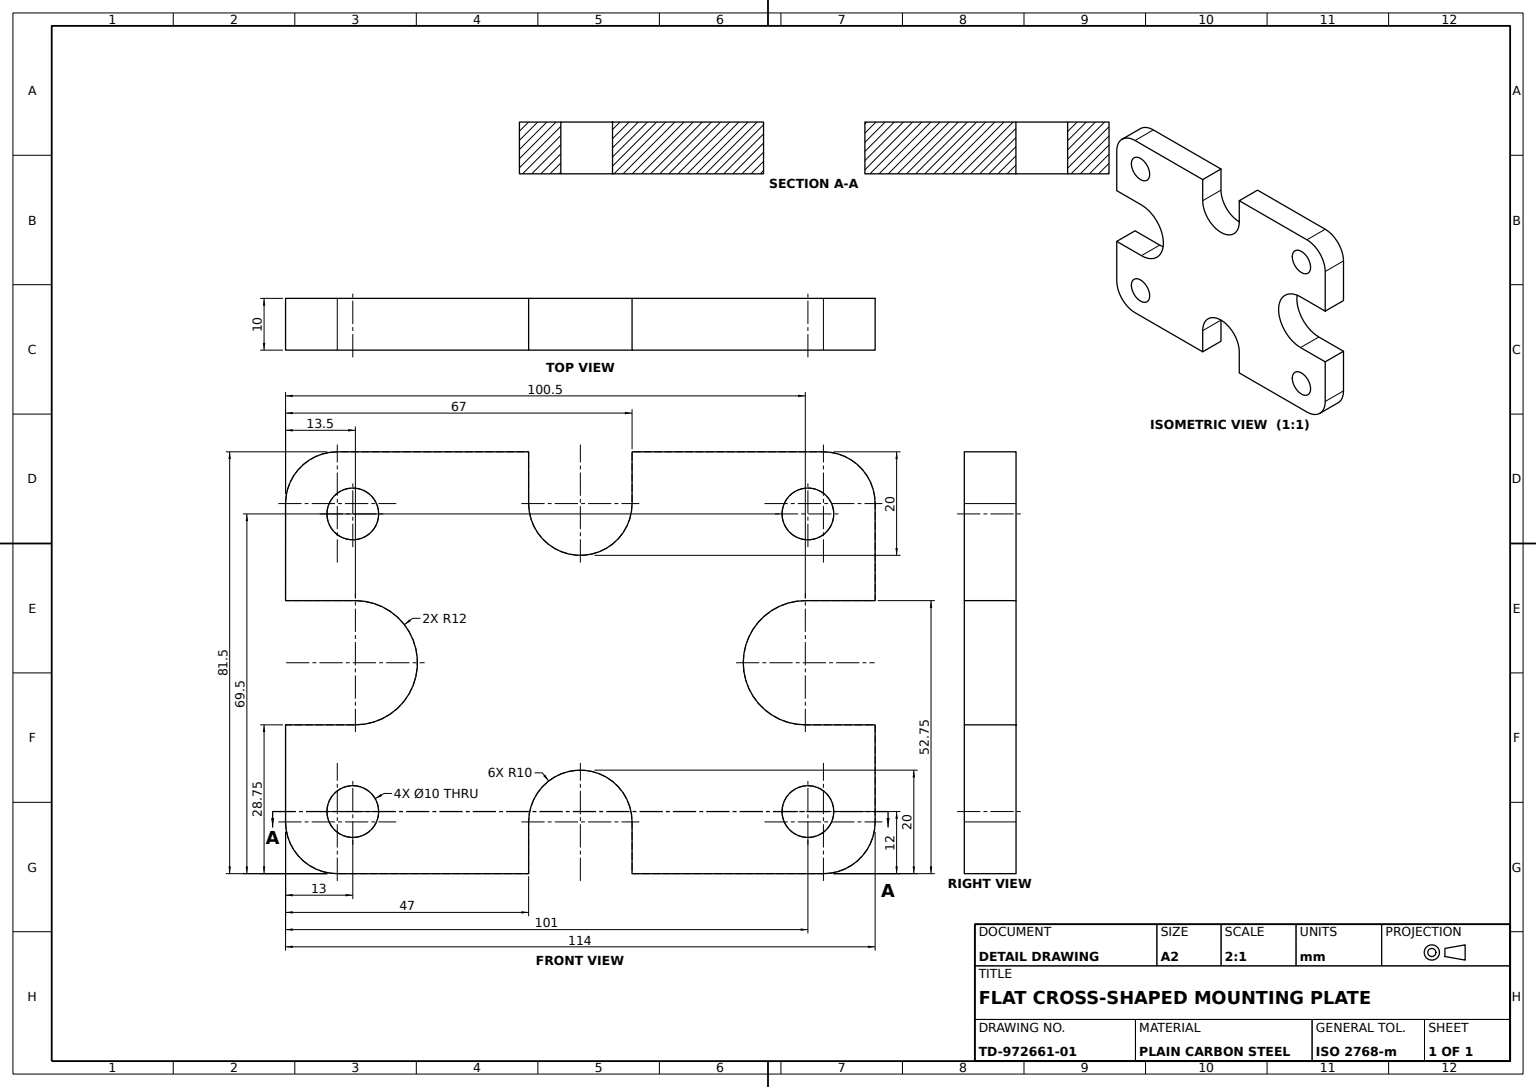
from build123d import *

# Parameters (mm, degrees)
BRACKET_PLATE_DEPTH        = 10
MOUNTING_HOLES_SKETCH_R    = 5
MOUNTING_HOLES_4X_10_DEPTH = 141.492882382
CORNER_FILLETS_R10_R       = 10


with BuildPart() as part:
    # Bracket Profile Sketch → Bracket Plate (new body)
    with BuildSketch(Plane.XY):
        with BuildLine():
            Line((10, 0), (47, 0))
            Line((47, 0), (47, 10))
            ThreePointArc((47, 10), (57, 20), (67, 10))
            Line((67, 10), (67, 0))
            Line((67, 0), (104, 0))
            Line((104, 0), (114, 0))
            Line((114, 0), (114, 10))
            Line((114, 10), (114, 28.75))
            Line((114, 28.75), (100.5, 28.75))
            ThreePointArc((100.5, 28.75), (88.5, 40.75), (100.5, 52.75))
            Line((100.5, 52.75), (114, 52.75))
            Line((114, 52.75), (114, 71.5))
            Line((114, 71.5), (114, 81.5))
            Line((114, 81.5), (104, 81.5))
            Line((104, 81.5), (67, 81.5))
            Line((67, 81.5), (67, 71.5))
            ThreePointArc((67, 71.5), (57, 61.5), (47, 71.5))
            Line((47, 71.5), (47, 81.5))
            Line((47, 81.5), (10, 81.5))
            Line((10, 81.5), (0, 81.5))
            Line((0, 81.5), (0, 71.5))
            Line((0, 71.5), (0, 52.75))
            Line((0, 52.75), (13.5, 52.75))
            ThreePointArc((13.5, 52.75), (25.5, 40.75), (13.5, 28.75))
            Line((13.5, 28.75), (0, 28.75))
            Line((0, 28.75), (0, 10))
            Line((0, 10), (0, 0))
            Line((0, 0), (10, 0))
        make_face()
    extrude(amount=BRACKET_PLATE_DEPTH)

    # Mounting Holes Sketch → Mounting Holes 4xØ10 (cut, through all)
    with BuildSketch(Plane.XY.offset(10)):
        with Locations((13, 69.5)):
            Circle(MOUNTING_HOLES_SKETCH_R)
        with Locations((101, 69.5)):
            Circle(MOUNTING_HOLES_SKETCH_R)
        with Locations((101, 12)):
            Circle(MOUNTING_HOLES_SKETCH_R)
        with Locations((13, 12)):
            Circle(MOUNTING_HOLES_SKETCH_R)
    extrude(amount=-MOUNTING_HOLES_4X_10_DEPTH, mode=Mode.SUBTRACT)

    # Corner Fillets R10
    corner_fillets_r10_edges = [part.edges().sort_by_distance(p)[0] for p in [
        (0, 0, 5),
        (0, 81.5, 5),
        (114, 81.5, 5),
        (114, 0, 5),
    ]]
    fillet(corner_fillets_r10_edges, radius=CORNER_FILLETS_R10_R)


solid = part.part
